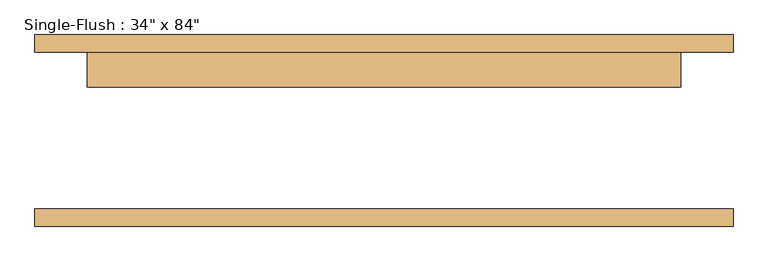
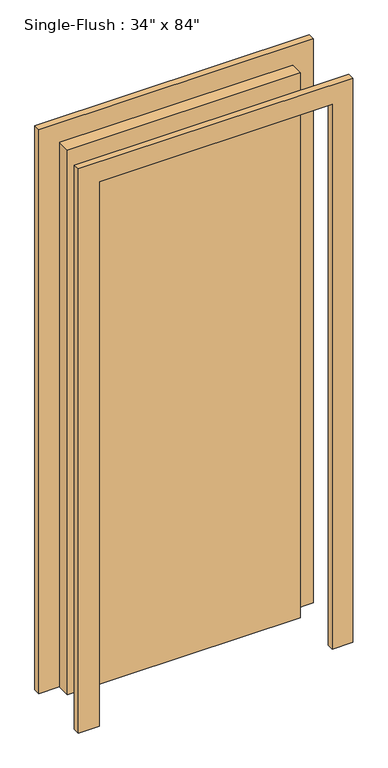
"""IFC4 building model written with IfcOpenShell, lengths in millimetres: door geometry."""

from ifc_helpers import new_model, si_unit, frame, origin, origin_with_axes, place, context, project, spatial, polyline, outline, extrude, source, transform, mapped, element, save


def door_de72ddbf(model_context):
    return source(origin(), model_context, "Body", "SweptSolid", [
        extrude(outline(polyline([(2209.8, -508.0), (0.0, -508.0), (0.0, -431.8), (2133.6, -431.8), (2133.6, 431.8), (0.0, 431.8), (0.0, 508.0), (2209.8, 508.0), (2209.8, -508.0)])), frame((0.0, 114.3, 0.0), z_axis=(0.0, 1.0, 0.0), x_axis=(0.0, 0.0, 1.0)), (0.0, 0.0, 1.0), 25.4),
        extrude(outline(polyline([(2209.8, 508.0), (2209.8, -508.0), (0.0, -508.0), (0.0, -431.8), (2133.6, -431.8), (2133.6, 431.8), (0.0, 431.8), (0.0, 508.0), (2209.8, 508.0)])), frame((0.0, -139.7, 0.0), z_axis=(0.0, 1.0, 0.0), x_axis=(0.0, 0.0, 1.0)), (0.0, 0.0, 1.0), 25.4),
        extrude(outline(polyline([(431.8, 63.5), (-431.8, 63.5), (-431.8, 114.3), (431.8, 114.3), (431.8, 63.5)])), origin_with_axes(), (0.0, 0.0, 1.0), 2133.6),
    ])


if __name__ == "__main__":
    model = new_model("IFC4")
    model_context = context("Model", 3, world=origin())
    ifc_project = project(units=[si_unit("LENGTHUNIT", "METRE", prefix="MILLI")], contexts=[model_context])
    site = spatial("IfcSite", under=ifc_project)
    building = spatial("IfcBuilding", under=site)
    placement = place(None, origin())
    door_shape = door_de72ddbf(model_context)
    element("IfcDoor", 1, ObjectType="Single-Flush : 34\" x 84\"", at=placement, inside=building, context=model_context, shape_type="MappedRepresentation", body=[
        mapped(door_shape, transform((0.0, 0.0, 0.0), x_axis=(1.0, 0.0, 0.0), y_axis=(0.0, 1.0, 0.0), z_axis=(0.0, 0.0, 1.0))),
    ])
    save(model, "model.ifc")

# Revit data of these elements
# Type "Single-Flush : 34\" x 84\""
#   Type Mark = "2"
#   Construction Type Id = "MDOOR"
#   Assembly Code = "C1020"
#   Analytic Construction = "Metal"
#   Thickness = 0' - 2"
#   Heat Transfer Coefficient (U) = 0.651978 BTU/(h·ft²·°F)
#   Height = 7' - 0"
#   Trim Projection Ext = 0' - 1"
#   Trim Projection Int = 0' - 1"
#   Trim Width = 0' - 3"
#   Width = 2' - 10"
#   Define Thermal Properties by = 1
#   Define Thermal Properties by = 1
#   Door Material = Door - Panel
#   Frame Material = Door - Frame
#   Visual Light Transmittance = 0
#   Solar Heat Gain Coefficient = 0
#   Function = (empty or 0)
#   Wall Closure = (empty or 0)
# Element 1 (IfcDoor, "Single-Flush : 34\" x 84\"")
#   Materials on its faces: "Door - Frame", "Door - Panel"
# Materials
#   "Door - Panel": class "Wood", colour RGB 210 159 95, transparency 0, Cost = 0
#   "Door - Frame": colour RGB 118 70 51, transparency 0, Cost = 0
